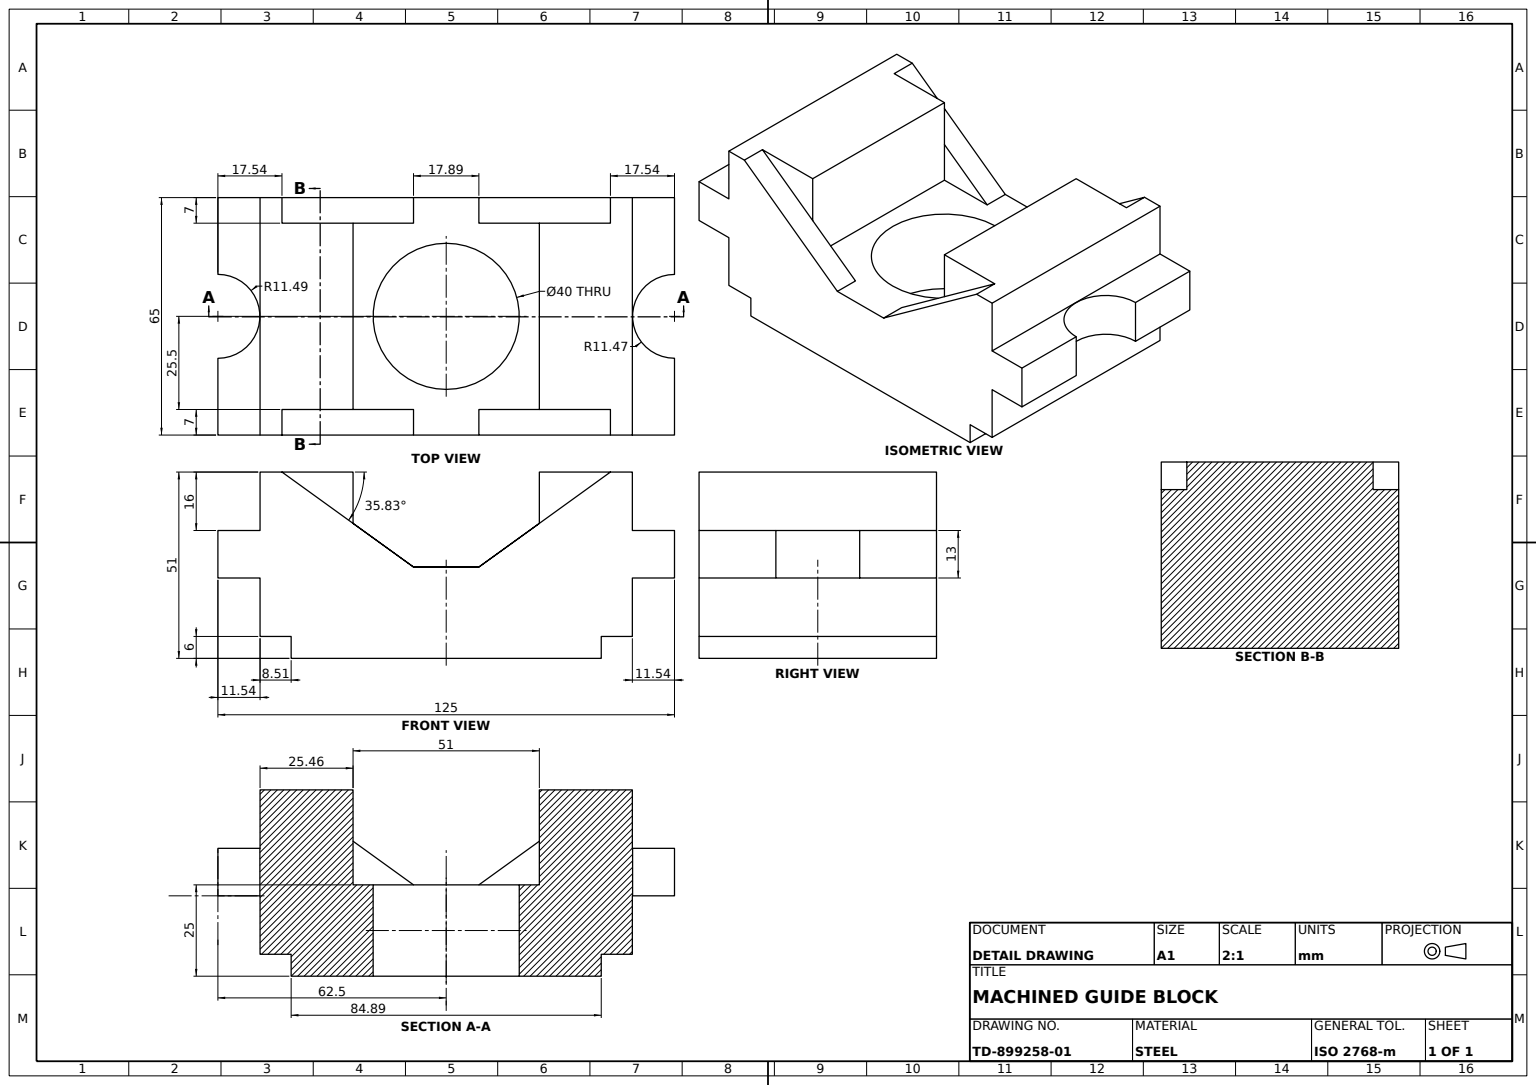
SolidWorks part; units mm, degrees
material "Plain Carbon Steel"
ref_plane "Front Plane" through (0, 0, 0) normal (0, 0, 1) x (1, 0, 0)
ref_plane "Top Plane" through (0, 0, 0) normal (0, 1, 0) x (1, 0, 0)
ref_plane "Right Plane" through (0, 0, 0) normal (1, 0, 0) x (0, 0, -1)
sketch "Stepped Cradle Profile Sketch" plane through (0, 0, 0) normal (0, 0, 1) x (1, 0, 0)
  line L1 (-42.4458, 0) -> (-42.4458, 6)
  line L2 (-42.4458, 6) -> (-50.9604, 6)
  line L3 (-50.9604, 6) -> (-50.9604, 22)
  line L4 (-50.9604, 22) -> (-62.5, 22)
  line L5 (-62.5, 22) -> (-62.5, 35)
  line L6 (-62.5, 35) -> (-50.9604, 35)
  line L7 (-50.9604, 35) -> (-50.9604, 51)
  line L8 (-50.9604, 51) -> (-44.9604, 51)
  line L11 (44.9604, 51) -> (8.9458, 25)
  line L12 (-8.9458, 0) -> (-42.4458, 0)
  line L13 (-44.9604, 51) -> (-8.9458, 25)
  line L14 (0, 25) -> (0, 47.2467) construction
  line L15 (8.9458, 0) -> (42.4458, 0)
  line L17 (50.9604, 51) -> (44.9604, 51)
  line L18 (50.9604, 35) -> (50.9604, 51)
  line L19 (62.5, 35) -> (50.9604, 35)
  line L20 (62.5, 22) -> (62.5, 35)
  line L21 (50.9604, 22) -> (62.5, 22)
  line L22 (50.9604, 6) -> (50.9604, 22)
  line L23 (42.4458, 6) -> (50.9604, 6)
  line L24 (42.4458, 0) -> (42.4458, 6)
  line L25 (-8.9458, 25) -> (8.9458, 25)
  line L26 (-8.9458, 0) -> (8.9458, 0)
  point P4 (1.5396, 0)
  dimension "D2" = 6
  dimension "D3" = 52.5
  dimension "D4" = 25
  dimension "D5" = 62.5
  dimension "D6" = 17.8916
  dimension "D7" = 6
  dimension "D8" = 33.5
  dimension "D9" = 11.5396
  dimension "D10" = 13
  dimension "D11" = 16
extrude "Stepped Cradle Block 65" add sketch "Stepped Cradle Profile Sketch" against normal blind 65 contours L13 L25 L11 L17 L18 L19 L20 L21 L22 L23 L24 L15 L26 L12 L1 L2 L3 L4 L5 L6 L7 L8
sketch "Raised Boss Sketch" plane through (0, 25, 0) normal (0, 1, 0) x (1, 0, 0)
  line L0 (-68.3121, 32.5) -> (70.113, 32.5) construction
  line L2 (-44.9604, 0) -> (-8.9458, 0) construction
  line L3 (-44.9604, 65) -> (-44.9604, 0) construction
  line L4 (-44.9604, 58) -> (-25.5, 58)
  line L5 (-44.9604, 58) -> (-44.9604, 7)
  line L6 (-44.9604, 7) -> (-25.5, 7)
  line L7 (-25.5, 58) -> (-25.5, 7)
  line L8 (0, 0) -> (0, 48.1112) construction
  line L9 (-8.9458, 0) -> (8.9458, 0) construction
  line L10 (44.9604, 7) -> (25.5, 7)
  line L11 (25.5, 58) -> (25.5, 7)
  line L12 (44.9604, 58) -> (44.9604, 7)
  line L13 (44.9604, 58) -> (25.5, 58)
  dimension "D1" = 32.5
  dimension "D2" = 25.5
  dimension "D3" = 25.5
  dimension "D4" = 25.5
extrude "Raised Boss" add sketch "Raised Boss Sketch" along normal up to surface (26 mm away) up to face at (-47.9604, 51, -32.5)
sketch "Cradle Slot Sketch" plane through (0, 25, 0) normal (0, 1, 0) x (1, 0, 0)
  line L1 (-25.5, 7) -> (25.5, 7)
  line L2 (-25.5, 7) -> (-25.5, 58)
  line L3 (-25.5, 58) -> (25.5, 58)
  line L4 (25.5, 7) -> (25.5, 58)
extrude "Cradle Slot Cut" cut sketch "Cradle Slot Sketch" along normal blind 41
sketch "Center Hole Sketch" plane through (0, 25, 0) normal (0, 1, 0) x (1, 0, 0)
  circle A0 centre (0, 32.5) radius 20
  dimension "D2" = 40
  dimension "D1" = 32.5
extrude "Center Hole Ø40" cut sketch "Center Hole Sketch" against normal blind 41
sketch "Front Relief Sketch" plane through (0, 35, 0) normal (0, 1, 0) x (1, 0, 0)
  line L0 (62.5, 65) -> (62.5, 0) construction
  line L1 (-62.5, 65) -> (-62.5, 0) construction
  circle A0 centre (62.5, 32.5) radius 11.4727
  circle A1 centre (-62.5, 32.5) radius 11.4918
  dimension "D1" = 22.9837
  dimension "D2" = 22.9454
extrude "Front Relief Cut" cut sketch "Front Relief Sketch" against normal blind 41
